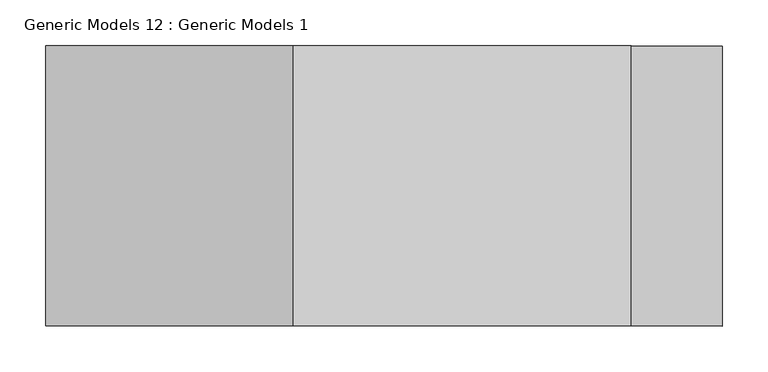
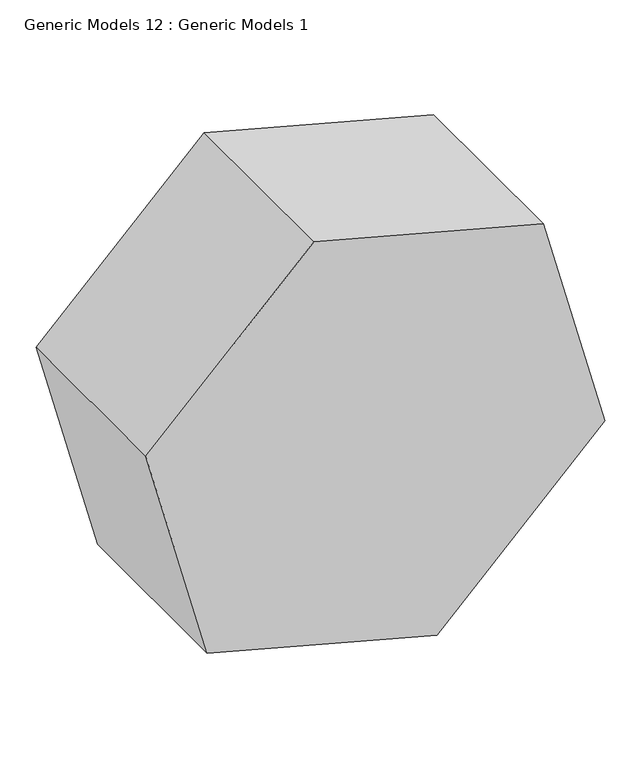
"""IFC4 building model written with IfcOpenShell, lengths in millimetres: proxy geometry, Generic Models 12 : Generic Models 1."""

from ifc_helpers import new_model, si_unit, frame, origin, place, context, project, spatial, polyline, outline, extrude, source, transform, mapped, element, save


def generic_models_12_generic_models_1_cd0b2d88(model_context):
    return source(origin(), model_context, "Body", "SweptSolid", [
        extrude(outline(polyline([(904.7566299, 3335.4198357), (1003.366686, 2967.4020959), (733.9590024, 2697.9944123), (365.9412626, 2796.6044685), (267.3312064, 3164.6222083), (536.73889, 3434.0298919), (904.7566299, 3335.4198357)])), frame((0.0, -9086.6225464, 0.0), z_axis=(0.0, 1.0, 0.0), x_axis=(0.0, 0.0, 1.0)), (0.0, 0.0, 1.0), 304.8),
    ])


if __name__ == "__main__":
    model = new_model("IFC4")
    model_context = context("Model", 3, world=origin())
    ifc_project = project(units=[si_unit("LENGTHUNIT", "METRE", prefix="MILLI")], contexts=[model_context])
    site = spatial("IfcSite", under=ifc_project)
    building = spatial("IfcBuilding", under=site)
    placement = place(None, origin())
    generic_models_12_generic_models_1_shape = generic_models_12_generic_models_1_cd0b2d88(model_context)
    element("IfcBuildingElementProxy", 1, Name="Generic Models 12 : Generic Models 1", ObjectType="Generic Models 12 : Generic Models 1", at=placement, inside=building, context=model_context, shape_type="MappedRepresentation", body=[
        mapped(generic_models_12_generic_models_1_shape, transform((0.0, 0.0, 0.0), x_axis=(1.0, 0.0, 0.0), y_axis=(0.0, 1.0, 0.0), z_axis=(0.0, 0.0, 1.0))),
    ])
    save(model, "model.ifc")

# Revit data of these elements
# Element 1 (IfcBuildingElementProxy, "Generic Models 12 : Generic Models 1")
#   Materials on its faces: "Brick, Common"
# Materials
#   "Brick, Common": class "Masonry", colour RGB 170 98 104, transparency 0, Description = "Common brick", Cost = 0
